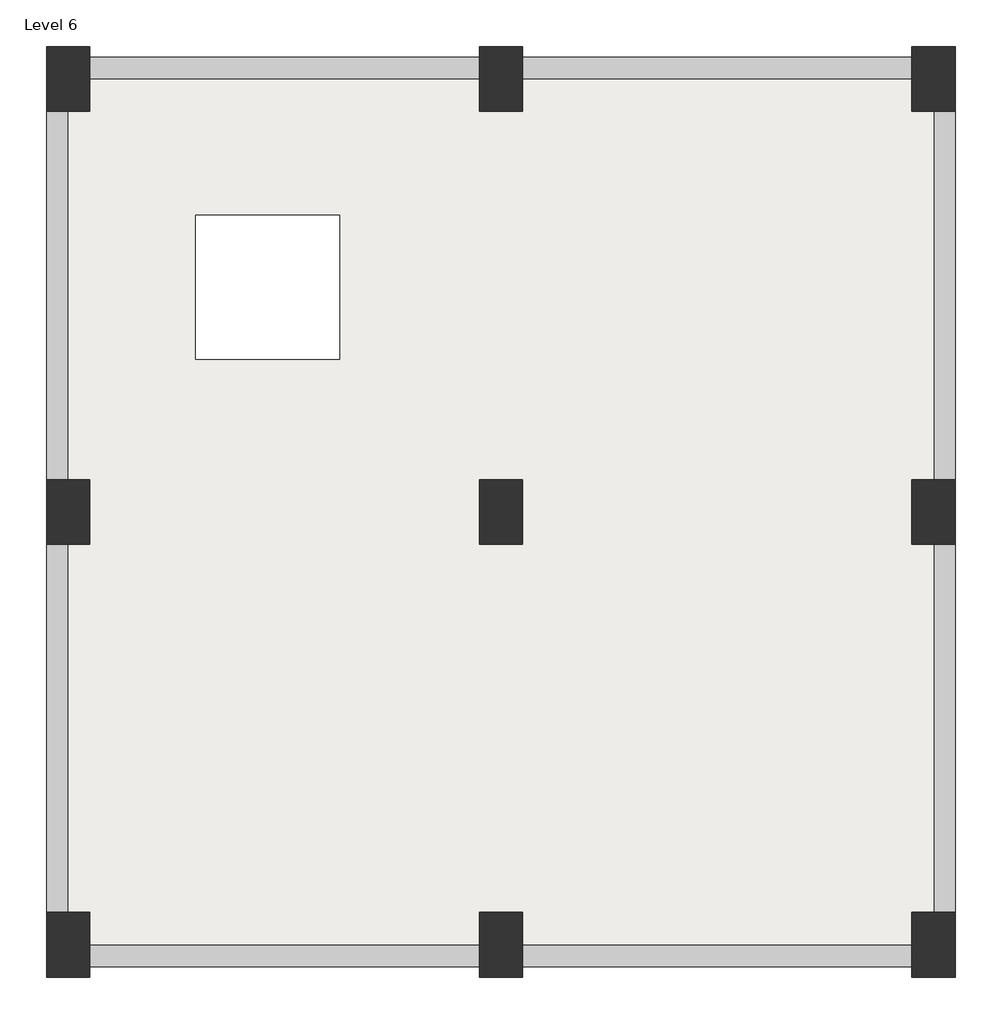
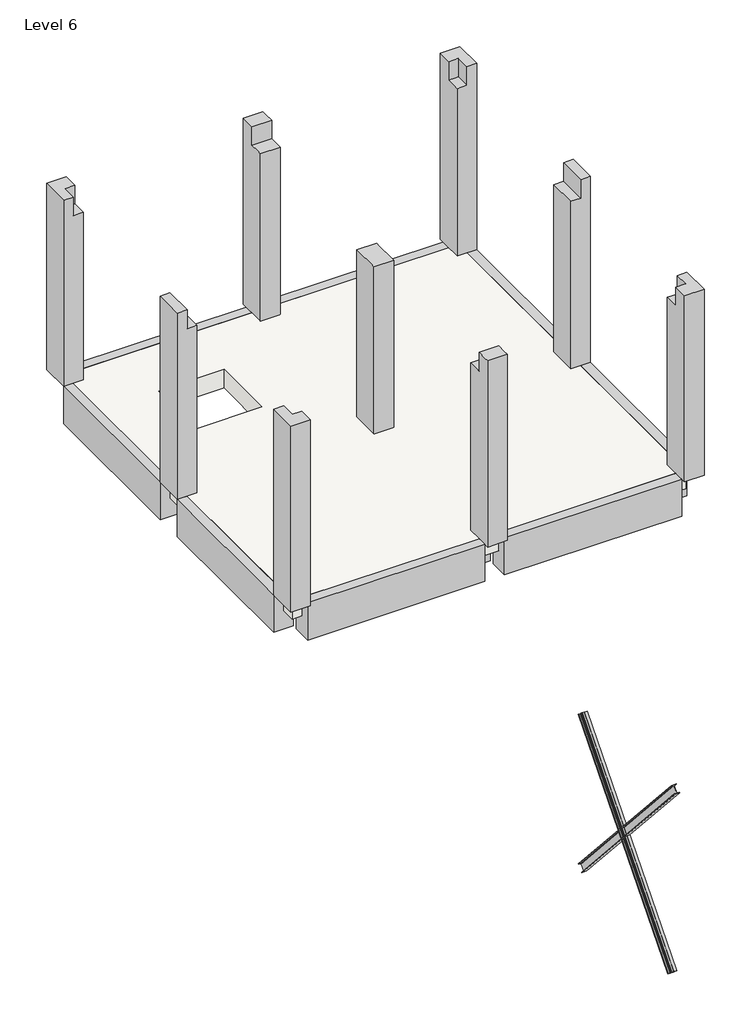
# One storey: 9 columns, 6 beams, 2 members, 1 slab.
"""IFC4 building model written with IfcOpenShell, lengths in millimetres."""

from ifc_helpers import new_model, si_unit, frame, origin, place, context, project, spatial, polyline, outline, extrude, faceted_brep, transform, mapped, element, save
from components import ub_universal_beams_ub127x76x13_58dc6553, ub_universal_beams_ub127x76x13_03bf5c3b

model = new_model("IFC4")

# Units and contexts
model_context = context("Model", 3, world=origin())
ifc_project = project(units=[si_unit("LENGTHUNIT", "METRE", prefix="MILLI")], contexts=[model_context])

# Site, building, storey
site = spatial("IfcSite", under=ifc_project)
building = spatial("IfcBuilding", under=site)
storey = spatial("IfcBuildingStorey", under=building, Name="Level 6", Elevation=15000.0)

# Beams
placement = place(None, origin())
element("IfcBeam", 1, ObjectType="Concrete-Rectangular Beam : 300 x 600mm", at=placement, inside=storey, context=model_context, shape_type="SweptSolid", body=[
    extrude(outline(polyline([(526.3372902, 14400.0), (226.3372902, 14400.0), (226.3372902, 14700.0), (376.3372902, 14700.0), (376.3372902, 15000.0), (526.3372902, 15000.0), (526.3372902, 14400.0)])), frame((2068.7595868, 0.0, 0.0), z_axis=(1.0, 0.0, 0.0), x_axis=(0.0, 1.0, 0.0)), (0.0, 0.0, 1.0), 2700.0),
    extrude(outline(polyline([(526.3372902, 14400.0), (226.3372902, 14400.0), (226.3372902, 14700.0), (376.3372902, 14700.0), (376.3372902, 15000.0), (526.3372902, 15000.0), (526.3372902, 14400.0)])), frame((-931.2404132, 0.0, 0.0), z_axis=(1.0, 0.0, 0.0), x_axis=(0.0, 1.0, 0.0)), (0.0, 0.0, 1.0), 2700.0),
])
element("IfcBeam", 2, ObjectType="Concrete-Rectangular Beam : 300 x 600mm", at=placement, inside=storey, context=model_context, shape_type="SweptSolid", body=[
    extrude(outline(polyline([(14400.0, 5068.7595868), (15000.0, 5068.7595868), (15000.0, 4918.7595868), (14700.0, 4918.7595868), (14700.0, 4768.7595868), (14400.0, 4768.7595868), (14400.0, 5068.7595868)])), frame((0.0, -2398.6627098, 0.0), z_axis=(0.0, 1.0, 0.0), x_axis=(0.0, 0.0, 1.0)), (0.0, 0.0, 1.0), 2550.0),
    extrude(outline(polyline([(14400.0, 5068.7595868), (15000.0, 5068.7595868), (15000.0, 4918.7595868), (14700.0, 4918.7595868), (14700.0, 4768.7595868), (14400.0, 4768.7595868), (14400.0, 5068.7595868)])), frame((0.0, -5398.6627098, 0.0), z_axis=(0.0, 1.0, 0.0), x_axis=(0.0, 0.0, 1.0)), (0.0, 0.0, 1.0), 2550.0),
])
element("IfcBeam", 3, ObjectType="Concrete-Rectangular Beam : 300 x 600mm", at=placement, inside=storey, context=model_context, shape_type="SweptSolid", body=[
    extrude(outline(polyline([(-5773.6627098, 14400.0), (-5773.6627098, 15000.0), (-5623.6627098, 15000.0), (-5623.6627098, 14700.0), (-5473.6627098, 14700.0), (-5473.6627098, 14400.0), (-5773.6627098, 14400.0)])), frame((2068.7595868, 0.0, 0.0), z_axis=(1.0, 0.0, 0.0), x_axis=(0.0, 1.0, 0.0)), (0.0, 0.0, 1.0), 2700.0),
    extrude(outline(polyline([(-5773.6627098, 14400.0), (-5773.6627098, 15000.0), (-5623.6627098, 15000.0), (-5623.6627098, 14700.0), (-5473.6627098, 14700.0), (-5473.6627098, 14400.0), (-5773.6627098, 14400.0)])), frame((-931.2404132, 0.0, 0.0), z_axis=(1.0, 0.0, 0.0), x_axis=(0.0, 1.0, 0.0)), (0.0, 0.0, 1.0), 2700.0),
])
element("IfcBeam", 4, ObjectType="Concrete-Rectangular Beam : 300 x 600mm", at=placement, inside=storey, context=model_context, shape_type="SweptSolid", body=[
    extrude(outline(polyline([(15000.0, -1231.2404132), (14400.0, -1231.2404132), (14400.0, -931.2404132), (14700.0, -931.2404132), (14700.0, -1081.2404132), (15000.0, -1081.2404132), (15000.0, -1231.2404132)])), frame((0.0, -5398.6627098, 0.0), z_axis=(0.0, 1.0, 0.0), x_axis=(0.0, 0.0, 1.0)), (0.0, 0.0, 1.0), 2550.0),
    extrude(outline(polyline([(15000.0, -1231.2404132), (14400.0, -1231.2404132), (14400.0, -931.2404132), (14700.0, -931.2404132), (14700.0, -1081.2404132), (15000.0, -1081.2404132), (15000.0, -1231.2404132)])), frame((0.0, -2398.6627098, 0.0), z_axis=(0.0, 1.0, 0.0), x_axis=(0.0, 0.0, 1.0)), (0.0, 0.0, 1.0), 2550.0),
])
element("IfcBeam", 5, ObjectType="Concrete-Rectangular Beam : 300 x 600mm", at=placement, inside=storey, context=model_context, shape_type="SweptSolid", body=[
    extrude(outline(polyline([(2068.7595868, -5398.6627098), (1768.7595868, -5398.6627098), (1768.7595868, -2848.6627098), (2068.7595868, -2848.6627098), (2068.7595868, -5398.6627098)])), frame((0.0, 0.0, 14400.0), z_axis=(0.0, 0.0, 1.0), x_axis=(1.0, 0.0, 0.0)), (0.0, 0.0, 1.0), 300.0),
    extrude(outline(polyline([(1768.7595868, 151.3372902), (2068.7595868, 151.3372902), (2068.7595868, -2398.6627098), (1768.7595868, -2398.6627098), (1768.7595868, 151.3372902)])), frame((0.0, 0.0, 14400.0), z_axis=(0.0, 0.0, 1.0), x_axis=(1.0, 0.0, 0.0)), (0.0, 0.0, 1.0), 300.0),
])
element("IfcBeam", 6, ObjectType="Concrete-Rectangular Beam : 300 x 600mm", at=placement, inside=storey, context=model_context, shape_type="SweptSolid", body=[
    extrude(outline(polyline([(4768.7595868, -2473.6627098), (4768.7595868, -2773.6627098), (2068.7595868, -2773.6627098), (2068.7595868, -2473.6627098), (4768.7595868, -2473.6627098)])), frame((0.0, 0.0, 14400.0), z_axis=(0.0, 0.0, 1.0), x_axis=(1.0, 0.0, 0.0)), (0.0, 0.0, 1.0), 300.0),
    extrude(outline(polyline([(-931.2404132, -2773.6627098), (-931.2404132, -2473.6627098), (1768.7595868, -2473.6627098), (1768.7595868, -2773.6627098), (-931.2404132, -2773.6627098)])), frame((0.0, 0.0, 14400.0), z_axis=(0.0, 0.0, 1.0), x_axis=(1.0, 0.0, 0.0)), (0.0, 0.0, 1.0), 300.0),
])

# Columns
element("IfcColumn", 7, ObjectType="Concrete-Rectangular-Column : 300 x 450mm", at=placement, inside=storey, context=model_context, shape_type="Brep", body=[
    faceted_brep([(-1231.2404132, -5848.6627098, 18000.0), (-931.2404132, -5848.6627098, 18000.0), (-931.2404132, -5623.6627098, 18000.0), (-1081.2404132, -5623.6627098, 18000.0), (-1081.2404132, -5398.6627098, 18000.0), (-1231.2404132, -5398.6627098, 18000.0), (-1231.2404132, -5848.6627098, 15000.0), (-1231.2404132, -5398.6627098, 15000.0), (-931.2404132, -5398.6627098, 15000.0), (-931.2404132, -5848.6627098, 15000.0), (-931.2404132, -5398.6627098, 17700.0), (-931.2404132, -5623.6627098, 17700.0), (-1081.2404132, -5398.6627098, 17700.0), (-1081.2404132, -5623.6627098, 17700.0)], [[[0, 1, 2, 3, 4, 5]], [[6, 7, 8, 9]], [[1, 0, 6, 9]], [[9, 8, 10, 11, 2, 1]], [[8, 7, 5, 4, 12, 10]], [[0, 5, 7, 6]], [[12, 13, 11, 10]], [[13, 3, 2, 11]], [[3, 13, 12, 4]]]),
])
element("IfcColumn", 8, ObjectType="Concrete-Rectangular-Column : 300 x 450mm", at=placement, inside=storey, context=model_context, shape_type="Brep", body=[
    faceted_brep([(1768.7595868, -5848.6627098, 18000.0), (2068.7595868, -5848.6627098, 18000.0), (2068.7595868, -5773.6627098, 18000.0), (2068.7595868, -5623.6627098, 18000.0), (1768.7595868, -5623.6627098, 18000.0), (1768.7595868, -5773.6627098, 18000.0), (1768.7595868, -5848.6627098, 15000.0), (1768.7595868, -5398.6627098, 15000.0), (2068.7595868, -5398.6627098, 15000.0), (2068.7595868, -5848.6627098, 15000.0), (2068.7595868, -5398.6627098, 17700.0), (2068.7595868, -5473.6627098, 17700.0), (2068.7595868, -5623.6627098, 17700.0), (1768.7595868, -5398.6627098, 17700.0), (1768.7595868, -5623.6627098, 17700.0), (1768.7595868, -5473.6627098, 17700.0)], [[[0, 1, 2, 3, 4, 5]], [[6, 7, 8, 9]], [[1, 0, 6, 9]], [[9, 8, 10, 11, 12, 3, 2, 1]], [[8, 7, 13, 10]], [[7, 6, 0, 5, 4, 14, 15, 13]], [[14, 12, 11, 10, 13, 15]], [[12, 14, 4, 3]]]),
])
element("IfcColumn", 9, ObjectType="Concrete-Rectangular-Column : 300 x 450mm", at=placement, inside=storey, context=model_context, shape_type="Brep", body=[
    faceted_brep([(4768.7595868, -5848.6627098, 18000.0), (5068.7595868, -5848.6627098, 18000.0), (5068.7595868, -5398.6627098, 18000.0), (4918.7595868, -5398.6627098, 18000.0), (4918.7595868, -5623.6627098, 18000.0), (4768.7595868, -5623.6627098, 18000.0), (4768.7595868, -5848.6627098, 15000.0), (4768.7595868, -5398.6627098, 15000.0), (5068.7595868, -5398.6627098, 15000.0), (5068.7595868, -5848.6627098, 15000.0), (4768.7595868, -5398.6627098, 17700.0), (4918.7595868, -5398.6627098, 17700.0), (4768.7595868, -5623.6627098, 17700.0), (4918.7595868, -5623.6627098, 17700.0)], [[[0, 1, 2, 3, 4, 5]], [[6, 7, 8, 9]], [[1, 0, 6, 9]], [[2, 1, 9, 8]], [[8, 7, 10, 11, 3, 2]], [[7, 6, 0, 5, 12, 10]], [[12, 13, 11, 10]], [[13, 4, 3, 11]], [[4, 13, 12, 5]]]),
])
element("IfcColumn", 10, ObjectType="Concrete-Rectangular-Column : 300 x 450mm", at=placement, inside=storey, context=model_context, shape_type="Brep", body=[
    faceted_brep([(-1231.2404132, -2398.6627098, 18000.0), (-1231.2404132, -2848.6627098, 18000.0), (-1081.2404132, -2848.6627098, 18000.0), (-1081.2404132, -2398.6627098, 18000.0), (-1231.2404132, -2848.6627098, 15000.0), (-1231.2404132, -2398.6627098, 15000.0), (-931.2404132, -2398.6627098, 15000.0), (-931.2404132, -2848.6627098, 15000.0), (-931.2404132, -2848.6627098, 17400.0), (-931.2404132, -2848.6627098, 17700.0), (-1081.2404132, -2848.6627098, 17700.0), (-1231.2404132, -2848.6627098, 17400.0), (-931.2404132, -2398.6627098, 17400.0), (-931.2404132, -2398.6627098, 17700.0), (-1231.2404132, -2398.6627098, 17400.0), (-1081.2404132, -2398.6627098, 17700.0)], [[[0, 1, 2, 3]], [[4, 5, 6, 7]], [[4, 7, 8, 9, 10, 2, 1, 11]], [[7, 6, 12, 13, 9, 8]], [[6, 5, 14, 0, 3, 15, 13, 12]], [[1, 0, 14, 5, 4, 11]], [[15, 10, 9, 13]], [[10, 15, 3, 2]]]),
])
element("IfcColumn", 11, ObjectType="Concrete-Rectangular-Column : 300 x 450mm", at=placement, inside=storey, context=model_context, shape_type="Brep", body=[
    faceted_brep([(1768.7595868, -2848.6627098, 15000.0), (1768.7595868, -2398.6627098, 15000.0), (2068.7595868, -2398.6627098, 15000.0), (2068.7595868, -2848.6627098, 15000.0), (2068.7595868, -2848.6627098, 17400.0), (2068.7595868, -2848.6627098, 17700.0), (1768.7595868, -2848.6627098, 17700.0), (1768.7595868, -2848.6627098, 17400.0), (2068.7595868, -2398.6627098, 17400.0), (2068.7595868, -2398.6627098, 17700.0), (2068.7595868, -2473.6627098, 17700.0), (2068.7595868, -2773.6627098, 17700.0), (1768.7595868, -2398.6627098, 17400.0), (1768.7595868, -2398.6627098, 17700.0), (1768.7595868, -2773.6627098, 17700.0), (1768.7595868, -2473.6627098, 17700.0)], [[[0, 1, 2, 3]], [[0, 3, 4, 5, 6, 7]], [[3, 2, 8, 9, 10, 11, 5, 4]], [[2, 1, 12, 13, 9, 8]], [[1, 0, 7, 6, 14, 15, 13, 12]], [[6, 5, 11, 10, 9, 13, 15, 14]]]),
])
element("IfcColumn", 12, ObjectType="Concrete-Rectangular-Column : 300 x 450mm", at=placement, inside=storey, context=model_context, shape_type="Brep", body=[
    faceted_brep([(5068.7595868, -2848.6627098, 18000.0), (5068.7595868, -2398.6627098, 18000.0), (4918.7595868, -2398.6627098, 18000.0), (4918.7595868, -2848.6627098, 18000.0), (4768.7595868, -2848.6627098, 15000.0), (4768.7595868, -2398.6627098, 15000.0), (5068.7595868, -2398.6627098, 15000.0), (5068.7595868, -2848.6627098, 15000.0), (5068.7595868, -2848.6627098, 17400.0), (4918.7595868, -2848.6627098, 17700.0), (4768.7595868, -2848.6627098, 17700.0), (4768.7595868, -2848.6627098, 17400.0), (5068.7595868, -2398.6627098, 17400.0), (4768.7595868, -2398.6627098, 17400.0), (4768.7595868, -2398.6627098, 17700.0), (4918.7595868, -2398.6627098, 17700.0)], [[[0, 1, 2, 3]], [[4, 5, 6, 7]], [[4, 7, 8, 0, 3, 9, 10, 11]], [[1, 0, 8, 7, 6, 12]], [[6, 5, 13, 14, 15, 2, 1, 12]], [[5, 4, 11, 10, 14, 13]], [[9, 15, 14, 10]], [[15, 9, 3, 2]]]),
])
element("IfcColumn", 13, ObjectType="Concrete-Rectangular-Column : 300 x 450mm", at=placement, inside=storey, context=model_context, shape_type="Brep", body=[
    faceted_brep([(-931.2404132, 601.3372902, 18000.0), (-1231.2404132, 601.3372902, 18000.0), (-1231.2404132, 151.3372902, 18000.0), (-1081.2404132, 151.3372902, 18000.0), (-1081.2404132, 376.3372902, 18000.0), (-931.2404132, 376.3372902, 18000.0), (-1231.2404132, 151.3372902, 15000.0), (-1231.2404132, 601.3372902, 15000.0), (-931.2404132, 601.3372902, 15000.0), (-931.2404132, 151.3372902, 15000.0), (-931.2404132, 151.3372902, 17700.0), (-1081.2404132, 151.3372902, 17700.0), (-931.2404132, 376.3372902, 17700.0), (-1081.2404132, 376.3372902, 17700.0)], [[[0, 1, 2, 3, 4, 5]], [[6, 7, 8, 9]], [[6, 9, 10, 11, 3, 2]], [[9, 8, 0, 5, 12, 10]], [[1, 0, 8, 7]], [[2, 1, 7, 6]], [[12, 13, 11, 10]], [[13, 4, 3, 11]], [[4, 13, 12, 5]]]),
])
element("IfcColumn", 14, ObjectType="Concrete-Rectangular-Column : 300 x 450mm", at=placement, inside=storey, context=model_context, shape_type="Brep", body=[
    faceted_brep([(2068.7595868, 601.3372902, 18000.0), (1768.7595868, 601.3372902, 18000.0), (1768.7595868, 526.3372902, 18000.0), (1768.7595868, 376.3372902, 18000.0), (2068.7595868, 376.3372902, 18000.0), (2068.7595868, 526.3372902, 18000.0), (1768.7595868, 151.3372902, 15000.0), (1768.7595868, 601.3372902, 15000.0), (2068.7595868, 601.3372902, 15000.0), (2068.7595868, 151.3372902, 15000.0), (2068.7595868, 151.3372902, 17700.0), (1768.7595868, 151.3372902, 17700.0), (2068.7595868, 376.3372902, 17700.0), (2068.7595868, 226.3372902, 17700.0), (1768.7595868, 226.3372902, 17700.0), (1768.7595868, 376.3372902, 17700.0)], [[[0, 1, 2, 3, 4, 5]], [[6, 7, 8, 9]], [[6, 9, 10, 11]], [[9, 8, 0, 5, 4, 12, 13, 10]], [[1, 0, 8, 7]], [[7, 6, 11, 14, 15, 3, 2, 1]], [[12, 15, 14, 11, 10, 13]], [[15, 12, 4, 3]]]),
])
element("IfcColumn", 15, ObjectType="Concrete-Rectangular-Column : 300 x 450mm", at=placement, inside=storey, context=model_context, shape_type="Brep", body=[
    faceted_brep([(5068.7595868, 151.3372902, 18000.0), (5068.7595868, 601.3372902, 18000.0), (4768.7595868, 601.3372902, 18000.0), (4768.7595868, 376.3372902, 18000.0), (4918.7595868, 376.3372902, 18000.0), (4918.7595868, 151.3372902, 18000.0), (4768.7595868, 151.3372902, 15000.0), (4768.7595868, 601.3372902, 15000.0), (5068.7595868, 601.3372902, 15000.0), (5068.7595868, 151.3372902, 15000.0), (4918.7595868, 151.3372902, 17700.0), (4768.7595868, 151.3372902, 17700.0), (4768.7595868, 376.3372902, 17700.0), (4918.7595868, 376.3372902, 17700.0)], [[[0, 1, 2, 3, 4, 5]], [[6, 7, 8, 9]], [[6, 9, 0, 5, 10, 11]], [[1, 0, 9, 8]], [[2, 1, 8, 7]], [[7, 6, 11, 12, 3, 2]], [[13, 12, 11, 10]], [[4, 13, 10, 5]], [[13, 4, 3, 12]]]),
])

# Members
ub_universal_beams_ub127x76x13_shape = ub_universal_beams_ub127x76x13_58dc6553(model_context)
element("IfcMember", 16, ObjectType="UB-Universal Beams : UB127x76x13", at=placement, inside=storey, context=model_context, shape_type="MappedRepresentation", body=[
    mapped(ub_universal_beams_ub127x76x13_shape, transform((4918.7595868, -3987.3365723, 8162.1128263), x_axis=(0.0, 0.665487731700438, -0.7464087881022075), y_axis=(-1.0, 0.0, 0.0), z_axis=(0.0, 0.7464087881022075, 0.665487731700438))),
])
ub_universal_beams_ub127x76x13_2_shape = ub_universal_beams_ub127x76x13_03bf5c3b(model_context)
element("IfcMember", 17, ObjectType="UB-Universal Beams : UB127x76x13", at=placement, inside=storey, context=model_context, shape_type="MappedRepresentation", body=[
    mapped(ub_universal_beams_ub127x76x13_2_shape, transform((4918.7595868, -3946.516498, 8229.9273511), x_axis=(0.0, -0.652009917674905, -0.7582104373151055), y_axis=(1.0, 0.0, 0.0), z_axis=(0.0, -0.7582104373151055, 0.652009917674905))),
])

# Slab
element("IfcSlab", 18, ObjectType="Generic 300mm", at=placement, inside=storey, context=model_context, shape_type="Brep", body=[
    faceted_brep([(4918.7595868, 376.3372902, 14700.0), (4918.7595868, 151.3372902, 14700.0), (4918.7595868, -2398.6627098, 14700.0), (4918.7595868, -2848.6627098, 14700.0), (4918.7595868, -5398.6627098, 14700.0), (4918.7595868, -5623.6627098, 14700.0), (4768.7595868, -5623.6627098, 14700.0), (2068.7595868, -5623.6627098, 14700.0), (1768.7595868, -5623.6627098, 14700.0), (-931.2404132, -5623.6627098, 14700.0), (-1081.2404132, -5623.6627098, 14700.0), (-1081.2404132, -5398.6627098, 14700.0), (-1081.2404132, -2848.6627098, 14700.0), (-1081.2404132, -2398.6627098, 14700.0), (-1081.2404132, 151.3372902, 14700.0), (-1081.2404132, 376.3372902, 14700.0), (-931.2404132, 376.3372902, 14700.0), (1768.7595868, 376.3372902, 14700.0), (2068.7595868, 376.3372902, 14700.0), (4768.7595868, 376.3372902, 14700.0), (-198.5229478, -1566.5574371, 14700.0), (801.4770522, -1566.5574371, 14700.0), (801.4770522, -566.5574371, 14700.0), (-198.5229478, -566.5574371, 14700.0), (4918.7595868, -5623.6627098, 15000.0), (4918.7595868, -5398.6627098, 15000.0), (4918.7595868, -2848.6627098, 15000.0), (4918.7595868, -2398.6627098, 15000.0), (4918.7595868, 151.3372902, 15000.0), (4918.7595868, 376.3372902, 15000.0), (4768.7595868, 376.3372902, 15000.0), (2068.7595868, 376.3372902, 15000.0), (1768.7595868, 376.3372902, 15000.0), (-931.2404132, 376.3372902, 15000.0), (-1081.2404132, 376.3372902, 15000.0), (-1081.2404132, 151.3372902, 15000.0), (-1081.2404132, -2398.6627098, 15000.0), (-1081.2404132, -2848.6627098, 15000.0), (-1081.2404132, -5398.6627098, 15000.0), (-1081.2404132, -5623.6627098, 15000.0), (-931.2404132, -5623.6627098, 15000.0), (1768.7595868, -5623.6627098, 15000.0), (2068.7595868, -5623.6627098, 15000.0), (4768.7595868, -5623.6627098, 15000.0), (801.4770522, -1566.5574371, 15000.0), (-198.5229478, -1566.5574371, 15000.0), (-198.5229478, -566.5574371, 15000.0), (801.4770522, -566.5574371, 15000.0)], [[[0, 1, 2, 3, 4, 5, 6, 7, 8, 9, 10, 11, 12, 13, 14, 15, 16, 17, 18, 19], [20, 21, 22, 23]], [[24, 25, 26, 27, 28, 29, 30, 31, 32, 33, 34, 35, 36, 37, 38, 39, 40, 41, 42, 43], [44, 45, 46, 47]], [[5, 4, 3, 2, 1, 0, 29, 28, 27, 26, 25, 24]], [[10, 9, 8, 7, 6, 5, 24, 43, 42, 41, 40, 39]], [[15, 14, 13, 12, 11, 10, 39, 38, 37, 36, 35, 34]], [[0, 19, 18, 17, 16, 15, 34, 33, 32, 31, 30, 29]], [[20, 45, 44, 21]], [[21, 44, 47, 22]], [[22, 47, 46, 23]], [[45, 20, 23, 46]]]),
])

save(model, "model.ifc")

# Revit data of these elements
# Type "Concrete-Rectangular Beam : 300 x 600mm"
#   Length [instance default] = 1.524 m
#   b = 0.3 m
#   h = 0.6 m
#   Structural Material [instance default] = Concrete, Cast-in-Place gray
#   Assembly Code = ""
# Type "Concrete-Rectangular-Column : 300 x 450mm"
#   b = 0.3 m
#   h = 0.45 m
#   Structural Material [instance default] = Concrete, Cast-in-Place gray
# Type "UB-Universal Beams : UB127x76x13"
#   Section Name Key = "UB127X76X13"
#   Width = 7.6 cm
#   Web Thickness = 0.4 cm
#   Web Fillet = 0.76 cm
#   Warping Constant = 2000.0 cm⁶
#   Torsional Moment of Inertia = 2.85 cm⁴
#   Section Area = 16.5 cm²
#   Plastic Modulus weak axis = 22.6 cm³
#   Plastic Modulus strong axis = 84.2 cm³
#   Nominal Weight = 13.00 kgf/m
#   Moment of Inertia weak axis = 55.70 cm⁴
#   Moment of Inertia strong axis = 473.00 cm⁴
#   Height = 12.7 cm
#   Flange Thickness = 0.76 cm
#   Elastic Modulus weak axis = 14.7 cm³
#   Elastic Modulus strong axis = 74.6 cm³
#   Centroid Vertical = 6.35 cm
#   Centroid Horizontal = 3.8 cm
#   Bolt Spacing = 4.0 cm
#   Length [instance default] = 1.5 m
#   Structural Material [instance default] = Metal - Steel 43-275
#   Type Comments = ""
#   Assembly Code = ""
# Type "Generic 300mm"
#   Function = 0
#   Layers, outside or top first: 0.3 m no material (function 1)
# Elements 1, 2, 3, 4, 5, 6 (IfcBeam, "Concrete-Rectangular Beam : 300 x 600mm")
#   Structural Material = Concrete, Cast-in-Place gray
#   Phase Created = New Construction
#   Materials on its faces: "Concrete, Cast-in-Place gray"
# Elements 7, 8, 9, 10, 11, 12, 13, 14, 15 (IfcColumn, "Concrete-Rectangular-Column : 300 x 450mm")
#   Structural Material = Concrete, Cast-in-Place gray
#   Phase Created = New Construction
#   Materials on its faces: "Concrete, Cast-in-Place gray"
# Elements 16, 17 (IfcMember, "UB-Universal Beams : UB127x76x13")
#   Structural Material = Metal - Steel 43-275
#   Phase Created = New Construction
#   Materials on its faces: "Metal - Steel 43-275"
# Element 18 (IfcSlab, "Generic 300mm")
#   Height Offset From Level = 0 m
#   built-in parameter 1001954 = 1
#   Phase Created = New Construction
#   Materials on its faces: "Default Floor"
# Materials
#   "Concrete, Cast-in-Place gray": class "Concrete", colour RGB 192 192 192, transparency 0, Description = "Cast-in-place concrete", Cost = 0
#   "Metal - Steel 43-275": class "Metal", colour RGB 247 247 247, transparency 0, Cost = 0
#   "Default Floor": colour RGB 127 127 127, transparency 0, Cost = 0
